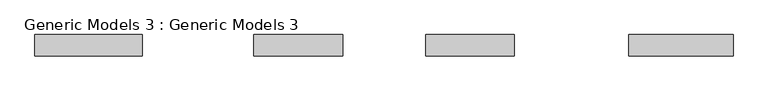
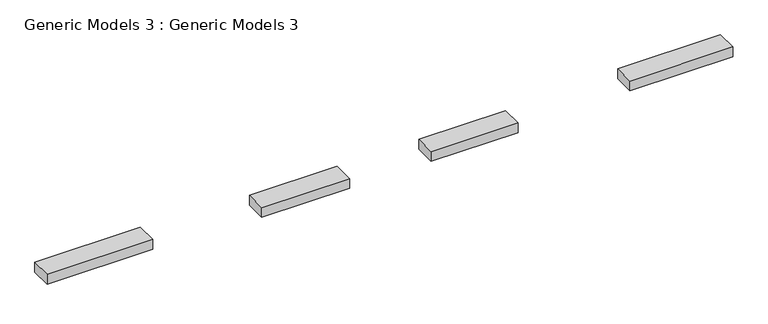
"""IFC4 building model written with IfcOpenShell, lengths in millimetres: proxy geometry, Generic Models 3 : Generic Models 3."""

from ifc_helpers import new_model, si_unit, frame, origin, place, context, project, spatial, polyline, outline, extrude, source, transform, mapped, element, save


def generic_models_3_generic_models_3_01e5b337(model_context):
    return source(origin(), model_context, "Body", "SweptSolid", [
        extrude(outline(polyline([(-6067.1942397, 8885.5272103), (-4578.5596144, 8885.5272103), (-4578.5596144, 8580.7272103), (-6067.1942397, 8580.7272103), (-6067.1942397, 8885.5272103)])), frame((0.0, 0.0, 2260.6), z_axis=(0.0, 0.0, 1.0), x_axis=(1.0, 0.0, 0.0)), (0.0, 0.0, 1.0), 152.4),
        extrude(outline(polyline([(-8952.7187727, 8885.5272103), (-7692.9270478, 8885.5272103), (-7692.9270478, 8580.7272103), (-8952.7187727, 8580.7272103), (-8952.7187727, 8885.5272103)])), frame((0.0, 0.0, 2190.75), z_axis=(0.0, 0.0, 1.0), x_axis=(1.0, 0.0, 0.0)), (0.0, 0.0, 1.0), 152.4),
        extrude(outline(polyline([(-11403.4518443, 8885.5272103), (-10134.7895677, 8885.5272103), (-10134.7895677, 8580.7272103), (-11403.4518443, 8580.7272103), (-11403.4518443, 8885.5272103)])), frame((0.0, 0.0, 2190.75), z_axis=(0.0, 0.0, 1.0), x_axis=(1.0, 0.0, 0.0)), (0.0, 0.0, 1.0), 152.4),
        extrude(outline(polyline([(-14517.0685074, 8885.5272103), (-12988.5597404, 8885.5272103), (-12988.5597404, 8580.7272103), (-14517.0685074, 8580.7272103), (-14517.0685074, 8885.5272103)])), frame((0.0, 0.0, 2260.6), z_axis=(0.0, 0.0, 1.0), x_axis=(1.0, 0.0, 0.0)), (0.0, 0.0, 1.0), 152.4),
    ])


if __name__ == "__main__":
    model = new_model("IFC4")
    model_context = context("Model", 3, world=origin())
    ifc_project = project(units=[si_unit("LENGTHUNIT", "METRE", prefix="MILLI")], contexts=[model_context])
    site = spatial("IfcSite", under=ifc_project)
    building = spatial("IfcBuilding", under=site)
    placement = place(None, origin())
    generic_models_3_generic_models_3_shape = generic_models_3_generic_models_3_01e5b337(model_context)
    element("IfcBuildingElementProxy", 1, Name="Generic Models 3 : Generic Models 3", ObjectType="Generic Models 3 : Generic Models 3", at=placement, inside=building, context=model_context, shape_type="MappedRepresentation", body=[
        mapped(generic_models_3_generic_models_3_shape, transform((0.0, 0.0, 0.0), x_axis=(1.0, 0.0, 0.0), y_axis=(0.0, 1.0, 0.0), z_axis=(0.0, 0.0, 1.0))),
    ])
    save(model, "model.ifc")
